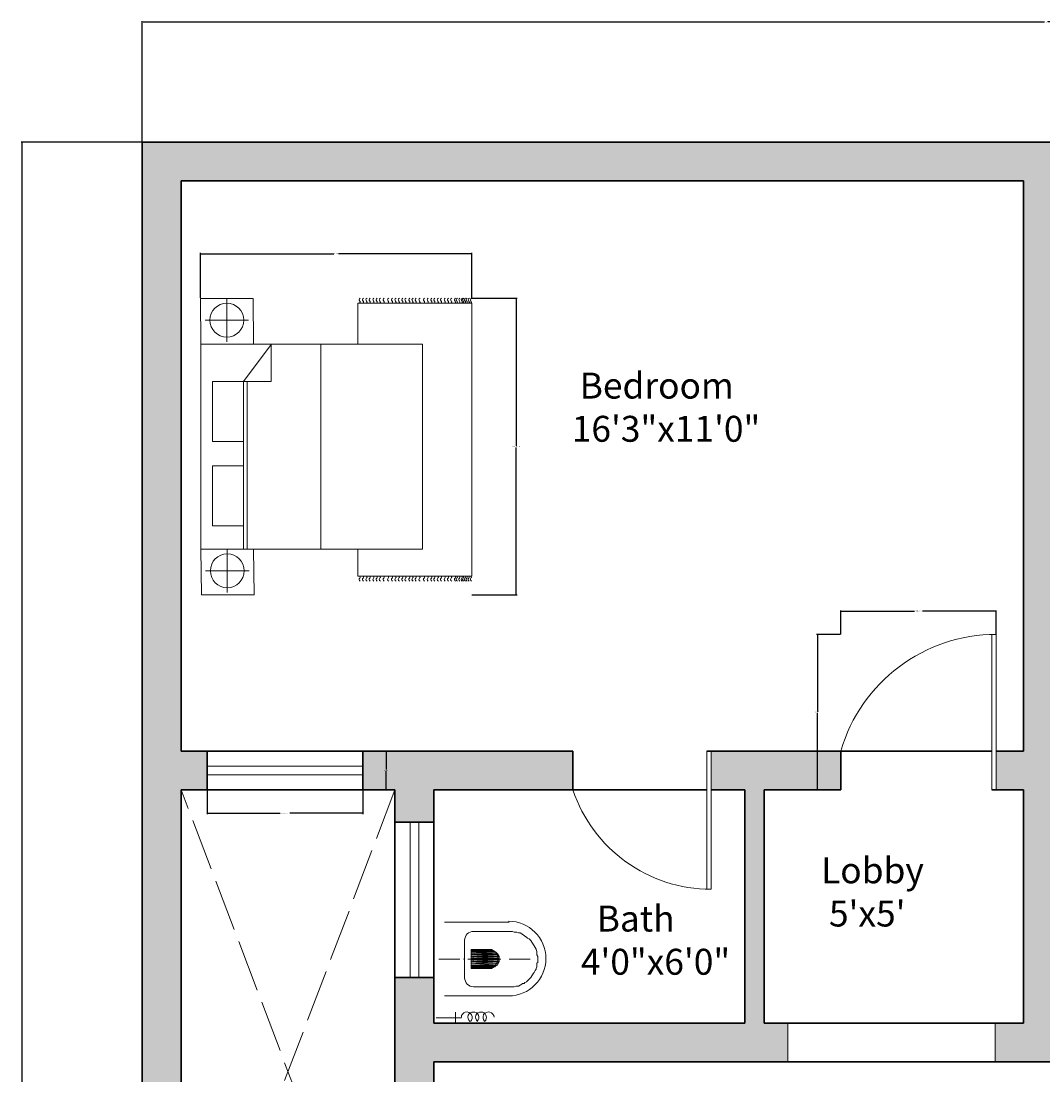
# Model space of a CAD drawing. Units: inches. Extents: x 1752 to 2227, y 6273 to 6884.
# Tile 5 of 6: x 1752 to 1989, y 6640 to 6884. Entities that reach past the tile are written whole.
import ezdxf

# ---------------------------------------------------------------- set-up
doc = ezdxf.new("R2010")
doc.units = ezdxf.units.IN
doc.header["$MEASUREMENT"] = 0
doc.linetypes.add('ACAD_ISO02W100', pattern=[15, 12, -3])
for name, color, linetype, lineweight in [('A-ANNO-DIMS', 2, 'Continuous', 18), ('A-AREA-IDEN', 7, 'Continuous', 18), ('A-DOOR', 3, 'Continuous', 20), ('A-FLOR-FIXT', 8, 'Continuous', 18), ('A-FLOR-VOID', 8, 'ACAD_ISO02W100', 13), ('A-FURN', 8, 'Continuous', 18), ('A-GLAZ', 4, 'Continuous', 18), ('A-WALL', 7, 'Continuous', 35), ('A-WALL-OPNG', 7, 'Continuous', 18)]:
    doc.layers.add(name, color=color, linetype=linetype, lineweight=lineweight)
doc.layers.add('A-WALL-PATT', color=32, linetype='Continuous', lineweight=13, true_color=0xcd6928)
doc.styles.get("Standard").update_dxf_attribs({"font": 'arial.ttf'})
doc.dimstyles.get("Standard").update_dxf_attribs({"dimtxt": 0.18, "dimasz": 0.18, "dimexe": 0.18, "dimexo": 0.0625, "dimgap": 0.09, "dimtad": 0, "dimtih": 1, "dimtoh": 1, "dimdec": 4, "dimzin": 0, "dimdsep": 46, "dimtxsty": 'Standard', "dimcen": 0.09, "dimadec": 0, "dimazin": 0, "dimtfac": 1, "dimtdec": 4, "dimtofl": 0, "dimtmove": 0, "dimatfit": 3, "dimfxl": 1, "dimtolj": 1, "dimtzin": 0, "dimarcsym": 0})

# ---------------------------------------------------------------- blocks, each defined once
blk = doc.blocks.new('BED-DOUBLE-SET')
for p, q in [((5.6, 61.62), (5.6, 51.56)), ((63.65, 61.72), (63.65, 51.66)), ((10.63, 56.59), (0.57, 56.59)), ((68.68, 56.69), (58.62, 56.69)), ((49.39, 52.82), (10.63, 52.82)), ((49.44, 52), (10.63, 52)), ((49.39, 52.82), (58, 46.47)), ((49.44, 52.82), (49.44, 46.47)), ((49.44, 46.47), (58, 46.47)), ((58.05, 34.96), (10.63, 34.96)), ((4.35, 0), (4.35, 26.37)), ((4.35, 26.37), (10.65, 26.37)), ((58.05, 26.37), (67.59, 26.37)), ((67.59, 26.37), (67.59, 0)), ((67.59, 0), (4.35, 0))]:
    blk.add_line(p, q)
for points in [[(0, 50.39), (10.63, 50.5), (10.63, 62.68), (0, 62.58)], [(58.05, 62.68), (58.05, 11.37), (10.63, 11.37), (10.63, 62.68)], [(58.05, 50.5), (68.68, 50.6), (68.68, 62.78), (58.05, 62.68)], [(29.88, 59.98), (29.88, 52.82), (15.98, 52.82), (15.98, 59.98)], [(49.44, 59.98), (49.44, 52.82), (35.55, 52.82), (35.55, 59.98)]]:
    blk.add_lwpolyline(points, close=True)
for centre in [(5.6, 56.59), (63.65, 56.69)]:
    blk.add_circle(centre, 3.92)
for points, knots in [([(3.23, 25.84), (3.32, 25.96), (3.52, 26.2), (3.86, 25.96), (4.14, 25.78), (4.29, 25.89), (4.35, 25.94)], [0, 0, 0, 0, 0.400747, 0.791423, 1.067667, 1.29709, 1.29709, 1.29709, 1.29709]), ([(3.23, 25.06), (3.32, 25.18), (3.52, 25.42), (3.86, 25.18), (4.14, 25.01), (4.29, 25.11), (4.35, 25.16)], [0, 0, 0, 0, 0.400747, 0.791423, 1.067667, 1.29709, 1.29709, 1.29709, 1.29709]), ([(3.23, 24.24), (3.32, 24.36), (3.52, 24.6), (3.86, 24.36), (4.14, 24.19), (4.29, 24.3), (4.35, 24.34)], [0, 0, 0, 0, 0.400747, 0.791423, 1.067667, 1.29709, 1.29709, 1.29709, 1.29709]), ([(68.71, 25.84), (68.61, 25.96), (68.42, 26.2), (68.08, 25.96), (67.8, 25.78), (67.65, 25.89), (67.58, 25.94)], [0, 0, 0, 0, 0.400747, 0.791423, 1.067667, 1.29709, 1.29709, 1.29709, 1.29709]), ([(68.71, 25.06), (68.61, 25.18), (68.42, 25.42), (68.08, 25.18), (67.8, 25.01), (67.65, 25.11), (67.58, 25.16)], [0, 0, 0, 0, 0.400747, 0.791423, 1.067667, 1.29709, 1.29709, 1.29709, 1.29709]), ([(68.71, 24.24), (68.61, 24.36), (68.42, 24.6), (68.08, 24.36), (67.8, 24.19), (67.65, 24.3), (67.58, 24.34)], [0, 0, 0, 0, 0.400747, 0.791423, 1.067667, 1.29709, 1.29709, 1.29709, 1.29709]), ([(3.23, 23.51), (3.32, 23.63), (3.52, 23.87), (3.86, 23.63), (4.14, 23.46), (4.29, 23.57), (4.35, 23.62)], [0, 0, 0, 0, 0.400747, 0.791423, 1.067667, 1.29709, 1.29709, 1.29709, 1.29709]), ([(3.23, 22.63), (3.32, 22.75), (3.52, 22.99), (3.86, 22.75), (4.14, 22.58), (4.29, 22.69), (4.35, 22.73)], [0, 0, 0, 0, 0.400747, 0.791423, 1.067667, 1.29709, 1.29709, 1.29709, 1.29709]), ([(3.23, 21.88), (3.32, 22), (3.52, 22.24), (3.86, 22), (4.14, 21.83), (4.29, 21.93), (4.35, 21.98)], [0, 0, 0, 0, 0.400747, 0.791423, 1.067667, 1.29709, 1.29709, 1.29709, 1.29709]), ([(68.71, 23.51), (68.61, 23.63), (68.42, 23.87), (68.08, 23.63), (67.8, 23.46), (67.65, 23.57), (67.58, 23.62)], [0, 0, 0, 0, 0.400747, 0.791423, 1.067667, 1.29709, 1.29709, 1.29709, 1.29709]), ([(68.71, 22.63), (68.61, 22.75), (68.42, 22.99), (68.08, 22.75), (67.8, 22.58), (67.65, 22.69), (67.58, 22.73)], [0, 0, 0, 0, 0.400747, 0.791423, 1.067667, 1.29709, 1.29709, 1.29709, 1.29709]), ([(68.71, 21.88), (68.61, 22), (68.42, 22.24), (68.08, 22), (67.8, 21.83), (67.65, 21.93), (67.58, 21.98)], [0, 0, 0, 0, 0.400747, 0.791423, 1.067667, 1.29709, 1.29709, 1.29709, 1.29709]), ([(3.23, 21.15), (3.32, 21.27), (3.52, 21.51), (3.86, 21.27), (4.14, 21.1), (4.29, 21.21), (4.35, 21.25)], [0, 0, 0, 0, 0.400747, 0.791423, 1.067667, 1.29709, 1.29709, 1.29709, 1.29709]), ([(3.23, 20.27), (3.32, 20.39), (3.52, 20.63), (3.86, 20.39), (4.14, 20.22), (4.29, 20.32), (4.35, 20.37)], [0, 0, 0, 0, 0.400747, 0.791423, 1.067667, 1.29709, 1.29709, 1.29709, 1.29709]), ([(68.71, 21.15), (68.61, 21.27), (68.42, 21.51), (68.08, 21.27), (67.8, 21.1), (67.65, 21.21), (67.58, 21.25)], [0, 0, 0, 0, 0.400747, 0.791423, 1.067667, 1.29709, 1.29709, 1.29709, 1.29709]), ([(68.71, 20.27), (68.61, 20.39), (68.42, 20.63), (68.08, 20.39), (67.8, 20.22), (67.65, 20.32), (67.58, 20.37)], [0, 0, 0, 0, 0.400747, 0.791423, 1.067667, 1.29709, 1.29709, 1.29709, 1.29709]), ([(3.23, 19.23), (3.32, 19.35), (3.52, 19.59), (3.86, 19.35), (4.14, 19.18), (4.29, 19.29), (4.35, 19.33)], [0, 0, 0, 0, 0.400747, 0.791423, 1.067667, 1.29709, 1.29709, 1.29709, 1.29709]), ([(3.23, 18.35), (3.32, 18.47), (3.52, 18.71), (3.86, 18.47), (4.14, 18.3), (4.29, 18.4), (4.35, 18.45)], [0, 0, 0, 0, 0.400747, 0.791423, 1.067667, 1.29709, 1.29709, 1.29709, 1.29709]), ([(3.23, 17.53), (3.32, 17.65), (3.52, 17.89), (3.86, 17.65), (4.14, 17.48), (4.29, 17.59), (4.35, 17.64)], [0, 0, 0, 0, 0.400747, 0.791423, 1.067667, 1.29709, 1.29709, 1.29709, 1.29709]), ([(68.71, 19.23), (68.61, 19.35), (68.42, 19.59), (68.08, 19.35), (67.8, 19.18), (67.65, 19.29), (67.58, 19.33)], [0, 0, 0, 0, 0.400747, 0.791423, 1.067667, 1.29709, 1.29709, 1.29709, 1.29709]), ([(68.71, 18.35), (68.61, 18.47), (68.42, 18.71), (68.08, 18.47), (67.8, 18.3), (67.65, 18.4), (67.58, 18.45)], [0, 0, 0, 0, 0.400747, 0.791423, 1.067667, 1.29709, 1.29709, 1.29709, 1.29709]), ([(68.71, 17.53), (68.61, 17.65), (68.42, 17.89), (68.08, 17.65), (67.8, 17.48), (67.65, 17.59), (67.58, 17.64)], [0, 0, 0, 0, 0.400747, 0.791423, 1.067667, 1.29709, 1.29709, 1.29709, 1.29709]), ([(3.23, 16.76), (3.32, 16.88), (3.52, 17.12), (3.86, 16.88), (4.14, 16.71), (4.29, 16.81), (4.35, 16.86)], [0, 0, 0, 0, 0.400747, 0.791423, 1.067667, 1.29709, 1.29709, 1.29709, 1.29709]), ([(3.23, 15.94), (3.32, 16.06), (3.52, 16.3), (3.86, 16.06), (4.14, 15.89), (4.29, 16), (4.35, 16.04)], [0, 0, 0, 0, 0.400747, 0.791423, 1.067667, 1.29709, 1.29709, 1.29709, 1.29709]), ([(3.23, 15.21), (3.32, 15.33), (3.52, 15.57), (3.86, 15.33), (4.14, 15.16), (4.29, 15.27), (4.35, 15.32)], [0, 0, 0, 0, 0.400747, 0.791423, 1.067667, 1.29709, 1.29709, 1.29709, 1.29709]), ([(68.71, 16.76), (68.61, 16.88), (68.42, 17.12), (68.08, 16.88), (67.8, 16.71), (67.65, 16.81), (67.58, 16.86)], [0, 0, 0, 0, 0.400747, 0.791423, 1.067667, 1.29709, 1.29709, 1.29709, 1.29709]), ([(68.71, 15.94), (68.61, 16.06), (68.42, 16.3), (68.08, 16.06), (67.8, 15.89), (67.65, 16), (67.58, 16.04)], [0, 0, 0, 0, 0.400747, 0.791423, 1.067667, 1.29709, 1.29709, 1.29709, 1.29709]), ([(68.71, 15.21), (68.61, 15.33), (68.42, 15.57), (68.08, 15.33), (67.8, 15.16), (67.65, 15.27), (67.58, 15.32)], [0, 0, 0, 0, 0.400747, 0.791423, 1.067667, 1.29709, 1.29709, 1.29709, 1.29709]), ([(3.23, 14.33), (3.32, 14.45), (3.52, 14.69), (3.86, 14.45), (4.14, 14.28), (4.29, 14.39), (4.35, 14.43)], [0, 0, 0, 0, 0.400747, 0.791423, 1.067667, 1.29709, 1.29709, 1.29709, 1.29709]), ([(3.23, 13.58), (3.32, 13.7), (3.52, 13.94), (3.86, 13.7), (4.14, 13.53), (4.29, 13.63), (4.35, 13.68)], [0, 0, 0, 0, 0.400747, 0.791423, 1.067667, 1.29709, 1.29709, 1.29709, 1.29709]), ([(3.23, 12.85), (3.32, 12.97), (3.52, 13.21), (3.86, 12.97), (4.14, 12.8), (4.29, 12.9), (4.35, 12.95)], [0, 0, 0, 0, 0.400747, 0.791423, 1.067667, 1.29709, 1.29709, 1.29709, 1.29709]), ([(3.23, 11.97), (3.32, 12.09), (3.52, 12.33), (3.86, 12.09), (4.14, 11.92), (4.29, 12.02), (4.35, 12.07)], [0, 0, 0, 0, 0.400747, 0.791423, 1.067667, 1.29709, 1.29709, 1.29709, 1.29709]), ([(68.71, 14.33), (68.61, 14.45), (68.42, 14.69), (68.08, 14.45), (67.8, 14.28), (67.65, 14.39), (67.58, 14.43)], [0, 0, 0, 0, 0.400747, 0.791423, 1.067667, 1.29709, 1.29709, 1.29709, 1.29709]), ([(68.71, 13.58), (68.61, 13.7), (68.42, 13.94), (68.08, 13.7), (67.8, 13.53), (67.65, 13.63), (67.58, 13.68)], [0, 0, 0, 0, 0.400747, 0.791423, 1.067667, 1.29709, 1.29709, 1.29709, 1.29709]), ([(68.71, 12.85), (68.61, 12.97), (68.42, 13.21), (68.08, 12.97), (67.8, 12.8), (67.65, 12.9), (67.58, 12.95)], [0, 0, 0, 0, 0.400747, 0.791423, 1.067667, 1.29709, 1.29709, 1.29709, 1.29709]), ([(68.71, 11.97), (68.61, 12.09), (68.42, 12.33), (68.08, 12.09), (67.8, 11.92), (67.65, 12.02), (67.58, 12.07)], [0, 0, 0, 0, 0.400747, 0.791423, 1.067667, 1.29709, 1.29709, 1.29709, 1.29709]), ([(3.23, 10.93), (3.32, 11.05), (3.52, 11.29), (3.86, 11.05), (4.14, 10.88), (4.29, 10.99), (4.35, 11.03)], [0, 0, 0, 0, 0.400747, 0.791423, 1.067667, 1.29709, 1.29709, 1.29709, 1.29709]), ([(3.23, 10.05), (3.32, 10.17), (3.52, 10.41), (3.86, 10.17), (4.14, 10), (4.29, 10.1), (4.35, 10.15)], [0, 0, 0, 0, 0.400747, 0.791423, 1.067667, 1.29709, 1.29709, 1.29709, 1.29709]), ([(68.71, 10.93), (68.61, 11.05), (68.42, 11.29), (68.08, 11.05), (67.8, 10.88), (67.65, 10.99), (67.58, 11.03)], [0, 0, 0, 0, 0.400747, 0.791423, 1.067667, 1.29709, 1.29709, 1.29709, 1.29709]), ([(68.71, 10.05), (68.61, 10.17), (68.42, 10.41), (68.08, 10.17), (67.8, 10), (67.65, 10.1), (67.58, 10.15)], [0, 0, 0, 0, 0.400747, 0.791423, 1.067667, 1.29709, 1.29709, 1.29709, 1.29709]), ([(3.23, 9.23), (3.32, 9.35), (3.52, 9.59), (3.86, 9.35), (4.14, 9.18), (4.29, 9.29), (4.35, 9.34)], [0, 0, 0, 0, 0.400747, 0.791423, 1.067667, 1.29709, 1.29709, 1.29709, 1.29709]), ([(3.23, 8.54), (3.32, 8.66), (3.52, 8.9), (3.86, 8.66), (4.14, 8.49), (4.29, 8.6), (4.35, 8.65)], [0, 0, 0, 0, 0.400747, 0.791423, 1.067667, 1.29709, 1.29709, 1.29709, 1.29709]), ([(3.23, 7.73), (3.32, 7.85), (3.52, 8.09), (3.86, 7.85), (4.14, 7.68), (4.29, 7.78), (4.35, 7.83)], [0, 0, 0, 0, 0.400747, 0.791423, 1.067667, 1.29709, 1.29709, 1.29709, 1.29709]), ([(68.71, 9.23), (68.61, 9.35), (68.42, 9.59), (68.08, 9.35), (67.8, 9.18), (67.65, 9.29), (67.58, 9.34)], [0, 0, 0, 0, 0.400747, 0.791423, 1.067667, 1.29709, 1.29709, 1.29709, 1.29709]), ([(68.71, 8.54), (68.61, 8.66), (68.42, 8.9), (68.08, 8.66), (67.8, 8.49), (67.65, 8.6), (67.58, 8.65)], [0, 0, 0, 0, 0.400747, 0.791423, 1.067667, 1.29709, 1.29709, 1.29709, 1.29709]), ([(68.71, 7.73), (68.61, 7.85), (68.42, 8.09), (68.08, 7.85), (67.8, 7.68), (67.65, 7.78), (67.58, 7.83)], [0, 0, 0, 0, 0.400747, 0.791423, 1.067667, 1.29709, 1.29709, 1.29709, 1.29709]), ([(3.23, 7), (3.32, 7.12), (3.52, 7.36), (3.86, 7.12), (4.14, 6.95), (4.29, 7.05), (4.35, 7.1)], [0, 0, 0, 0, 0.400747, 0.791423, 1.067667, 1.29709, 1.29709, 1.29709, 1.29709]), ([(3.23, 6.12), (3.32, 6.24), (3.52, 6.48), (3.86, 6.24), (4.14, 6.07), (4.29, 6.17), (4.35, 6.22)], [0, 0, 0, 0, 0.400747, 0.791423, 1.067667, 1.29709, 1.29709, 1.29709, 1.29709]), ([(3.23, 5.37), (3.32, 5.49), (3.52, 5.73), (3.86, 5.49), (4.14, 5.31), (4.29, 5.42), (4.35, 5.47)], [0, 0, 0, 0, 0.400747, 0.791423, 1.067667, 1.29709, 1.29709, 1.29709, 1.29709]), ([(3.23, 4.64), (3.32, 4.76), (3.52, 5), (3.86, 4.76), (4.14, 4.59), (4.29, 4.69), (4.35, 4.74)], [0, 0, 0, 0, 0.400747, 0.791423, 1.067667, 1.29709, 1.29709, 1.29709, 1.29709]), ([(68.71, 7), (68.61, 7.12), (68.42, 7.36), (68.08, 7.12), (67.8, 6.95), (67.65, 7.05), (67.58, 7.1)], [0, 0, 0, 0, 0.400747, 0.791423, 1.067667, 1.29709, 1.29709, 1.29709, 1.29709]), ([(68.71, 6.12), (68.61, 6.24), (68.42, 6.48), (68.08, 6.24), (67.8, 6.07), (67.65, 6.17), (67.58, 6.22)], [0, 0, 0, 0, 0.400747, 0.791423, 1.067667, 1.29709, 1.29709, 1.29709, 1.29709]), ([(68.71, 5.37), (68.61, 5.49), (68.42, 5.73), (68.08, 5.49), (67.8, 5.31), (67.65, 5.42), (67.58, 5.47)], [0, 0, 0, 0, 0.400747, 0.791423, 1.067667, 1.29709, 1.29709, 1.29709, 1.29709]), ([(68.71, 4.64), (68.61, 4.76), (68.42, 5), (68.08, 4.76), (67.8, 4.59), (67.66, 4.69), (67.59, 4.73)], [0, 0, 0, 0, 0.400747, 0.791423, 1.067667, 1.283686, 1.283686, 1.283686, 1.283686]), ([(3.23, 3.75), (3.32, 3.88), (3.52, 4.12), (3.86, 3.88), (4.14, 3.7), (4.29, 3.81), (4.35, 3.86)], [0, 0, 0, 0, 0.400747, 0.791423, 1.067667, 1.29709, 1.29709, 1.29709, 1.29709]), ([(3.23, 3.33), (3.32, 3.45), (3.52, 3.7), (3.86, 3.45), (4.14, 3.27), (4.29, 3.38), (4.35, 3.43)], [0, 0, 0, 0, 0.407265, 0.802015, 1.07826, 1.307683, 1.307683, 1.307683, 1.307683]), ([(3.23, 2.76), (3.32, 2.88), (3.52, 3.12), (3.86, 2.88), (4.14, 2.71), (4.29, 2.81), (4.35, 2.86)], [0, 0, 0, 0, 0.400747, 0.791423, 1.067667, 1.29709, 1.29709, 1.29709, 1.29709]), ([(3.23, 2.19), (3.32, 2.31), (3.52, 2.55), (3.86, 2.31), (4.14, 2.13), (4.29, 2.24), (4.35, 2.29)], [0, 0, 0, 0, 0.400747, 0.791423, 1.067667, 1.29709, 1.29709, 1.29709, 1.29709]), ([(68.71, 3.75), (68.61, 3.88), (68.42, 4.12), (68.08, 3.88), (67.8, 3.7), (67.66, 3.81), (67.59, 3.85)], [0, 0, 0, 0, 0.400747, 0.791423, 1.067667, 1.283686, 1.283686, 1.283686, 1.283686]), ([(68.71, 3.33), (68.61, 3.45), (68.42, 3.69), (68.08, 3.45), (67.8, 3.28), (67.66, 3.38), (67.59, 3.42)], [0, 0, 0, 0, 0.402903, 0.794912, 1.071156, 1.287177, 1.287177, 1.287177, 1.287177]), ([(68.71, 2.73), (68.61, 2.85), (68.42, 3.09), (68.08, 2.85), (67.8, 2.68), (67.66, 2.78), (67.59, 2.83)], [0, 0, 0, 0, 0.400747, 0.791423, 1.067667, 1.283686, 1.283686, 1.283686, 1.283686]), ([(3.23, 1.88), (3.32, 2), (3.52, 2.24), (3.86, 2), (4.14, 1.82), (4.29, 1.93), (4.35, 1.98)], [0, 0, 0, 0, 0.400747, 0.791423, 1.067667, 1.29709, 1.29709, 1.29709, 1.29709]), ([(3.23, 1.46), (3.32, 1.58), (3.52, 1.82), (3.86, 1.58), (4.14, 1.41), (4.29, 1.51), (4.35, 1.56)], [0, 0, 0, 0, 0.400747, 0.791423, 1.067667, 1.29709, 1.29709, 1.29709, 1.29709]), ([(3.23, 1.06), (3.32, 1.18), (3.52, 1.42), (3.86, 1.18), (4.14, 1.01), (4.29, 1.11), (4.35, 1.16)], [0, 0, 0, 0, 0.400747, 0.791423, 1.067667, 1.29709, 1.29709, 1.29709, 1.29709]), ([(3.23, 0.57), (3.32, 0.7), (3.52, 0.94), (3.86, 0.7), (4.14, 0.52), (4.29, 0.63), (4.35, 0.68)], [0, 0, 0, 0, 0.400747, 0.791423, 1.067667, 1.29709, 1.29709, 1.29709, 1.29709]), ([(3.23, 0.07), (3.32, 0.19), (3.52, 0.43), (3.86, 0.19), (4.14, 0.02), (4.29, 0.13), (4.35, 0.18)], [0, 0, 0, 0, 0.400747, 0.791423, 1.067667, 1.29709, 1.29709, 1.29709, 1.29709]), ([(68.71, 1.43), (68.61, 1.55), (68.42, 1.79), (68.08, 1.55), (67.8, 1.38), (67.65, 1.48), (67.58, 1.53)], [0, 0, 0, 0, 0.400747, 0.791423, 1.067667, 1.29709, 1.29709, 1.29709, 1.29709]), ([(68.71, 1.03), (68.61, 1.15), (68.42, 1.39), (68.08, 1.15), (67.8, 0.98), (67.65, 1.09), (67.58, 1.13)], [0, 0, 0, 0, 0.400747, 0.791423, 1.067667, 1.29709, 1.29709, 1.29709, 1.29709]), ([(68.71, 0.55), (68.61, 0.67), (68.42, 0.91), (68.08, 0.67), (67.8, 0.5), (67.65, 0.6), (67.58, 0.65)], [0, 0, 0, 0, 0.400747, 0.791423, 1.067667, 1.29709, 1.29709, 1.29709, 1.29709]), ([(68.71, 0.07), (68.61, 0.19), (68.42, 0.43), (68.08, 0.19), (67.8, 0.02), (67.65, 0.13), (67.58, 0.18)], [0, 0, 0, 0, 0.400747, 0.791423, 1.067667, 1.29709, 1.29709, 1.29709, 1.29709]), ([(68.71, 2.16), (68.61, 2.28), (68.42, 2.52), (68.08, 2.28), (67.8, 2.11), (67.66, 2.21), (67.59, 2.25)], [0, 0, 0, 0, 0.400747, 0.791423, 1.067667, 1.283686, 1.283686, 1.283686, 1.283686]), ([(68.71, 1.85), (68.61, 1.97), (68.42, 2.21), (68.08, 1.97), (67.8, 1.8), (67.66, 1.9), (67.59, 1.94)], [0, 0, 0, 0, 0.400747, 0.791423, 1.067667, 1.283686, 1.283686, 1.283686, 1.283686])]:
    blk.add_open_spline(points, degree=3, knots=knots)
blk = doc.blocks.new('WC-PLAN')
h = blk.add_hatch(color=256)
h.paths.add_polyline_path([(8.12, 16.94), (13.2, 16.94), (8.12, 17.17)])
h.paths.add_polyline_path([(13.2, 16.94), (8.12, 17.17), (12.82, 17.17)])
h.paths.add_polyline_path([(8.12, 17.17), (12.82, 17.17), (12.44, 17.17)])
h = blk.add_hatch(color=256)
h.paths.add_polyline_path([(8.12, 16.71), (13.58, 16.71), (8.12, 16.94)])
h.paths.add_polyline_path([(13.58, 16.71), (8.12, 16.94), (13.2, 16.94)])
h = blk.add_hatch(color=256)
h.paths.add_polyline_path([(8.12, 16.56), (13.81, 16.56), (8.12, 16.71)])
h.paths.add_polyline_path([(13.81, 16.56), (8.12, 16.71), (13.58, 16.71)])
h = blk.add_hatch(color=256)
h.paths.add_polyline_path([(8.12, 16.18), (14.19, 16.18), (8.12, 16.56)])
h.paths.add_polyline_path([(14.19, 16.18), (8.12, 16.56), (13.81, 16.56)])
h = blk.add_hatch(color=256)
h.paths.add_polyline_path([(8.12, 15.95), (14.34, 15.95), (8.12, 16.18)])
h.paths.add_polyline_path([(14.34, 15.95), (8.12, 16.18), (14.19, 16.18)])
h = blk.add_hatch(color=256)
h.paths.add_polyline_path([(8.12, 15.57), (14.56, 15.57), (8.12, 15.95)])
h.paths.add_polyline_path([(14.56, 15.57), (8.12, 15.95), (14.34, 15.95)])
h = blk.add_hatch(color=256)
h.paths.add_polyline_path([(8.12, 15.19), (14.56, 15.19), (8.12, 15.57)])
h.paths.add_polyline_path([(14.56, 15.19), (8.12, 15.57), (14.56, 15.57)])
h = blk.add_hatch(color=256)
h.paths.add_polyline_path([(8.12, 14.81), (14.56, 14.81), (8.12, 15.19)])
h.paths.add_polyline_path([(14.56, 14.81), (8.12, 15.19), (14.56, 15.19)])
h = blk.add_hatch(color=256)
h.paths.add_polyline_path([(8.12, 14.44), (14.56, 14.44), (8.12, 14.81)])
h.paths.add_polyline_path([(14.56, 14.44), (8.12, 14.81), (14.56, 14.81)])
h = blk.add_hatch(color=256)
h.paths.add_polyline_path([(8.12, 14.06), (14.34, 14.06), (8.12, 14.44)])
h.paths.add_polyline_path([(14.34, 14.06), (8.12, 14.44), (14.56, 14.44)])
h = blk.add_hatch(color=256)
h.paths.add_polyline_path([(8.12, 13.6), (14.19, 13.6), (8.12, 14.06)])
h.paths.add_polyline_path([(14.19, 13.6), (8.12, 14.06), (14.34, 14.06)])
h = blk.add_hatch(color=256)
h.paths.add_polyline_path([(8.12, 13.45), (13.81, 13.45), (8.12, 13.6)])
h.paths.add_polyline_path([(13.81, 13.45), (8.12, 13.6), (14.19, 13.6)])
h = blk.add_hatch(color=256)
h.paths.add_polyline_path([(8.12, 13.22), (13.58, 13.22), (8.12, 13.45)])
h.paths.add_polyline_path([(13.58, 13.22), (8.12, 13.45), (13.81, 13.45)])
h = blk.add_hatch(color=256)
h.paths.add_polyline_path([(8.12, 13.07), (13.2, 13.07), (8.12, 13.22)])
h.paths.add_polyline_path([(13.2, 13.07), (8.12, 13.22), (13.58, 13.22)])
h = blk.add_hatch(color=256)
h.paths.add_polyline_path([(8.12, 12.84), (12.82, 12.84), (8.12, 13.07)])
h.paths.add_polyline_path([(12.82, 12.84), (8.12, 13.07), (13.2, 13.07)])
for points in [[(1.9, 23.54), (16.92, 23.54), (16.92, 23.54)], [(8.72, 21.41), (15.93, 21.41), (15.93, 21.41)], [(15.93, 21.41), (16.69, 21.41), (17.3, 21.41), (17.67, 21.41), (18.05, 21.19), (18.43, 21.19), (18.66, 21.19), (19.04, 21.04), (19.42, 21.04), (19.8, 20.81), (20.03, 20.66), (20.41, 20.43), (20.56, 20.28), (20.94, 20.05), (21.16, 19.82), (21.54, 19.67), (21.77, 19.44), (21.92, 19.29), (22.15, 18.91), (22.3, 18.68), (22.53, 18.3), (22.68, 18.08), (22.91, 17.7), (23.14, 17.32), (23.14, 17.17), (23.29, 16.71), (23.29, 16.33), (23.29, 15.95), (23.52, 15.57), (23.52, 14.97), (23.52, 14.21), (23.29, 14.06), (23.29, 13.6), (23.29, 13.22), (23.14, 12.84), (23.14, 12.69), (22.91, 12.31), (22.68, 11.86), (22.53, 11.7), (22.3, 11.33), (22.15, 11.1), (21.92, 10.72), (21.77, 10.57), (21.54, 10.34), (21.16, 9.96), (20.94, 9.73), (20.56, 9.58), (20.41, 9.35), (20.03, 9.35), (19.8, 9.2), (19.42, 8.97), (19.04, 8.75), (18.66, 8.75), (18.43, 8.75), (18.05, 8.59), (17.67, 8.59), (17.3, 8.59), (16.69, 8.59), (15.93, 8.59)], [(6.6, 19.29), (6.6, 10.57), (6.6, 10.57)], [(8.12, 17.17), (8.12, 12.84), (8.12, 12.84)], [(8.12, 17.17), (12.44, 17.17), (12.44, 17.17)], [(0.61, 14.97), (5.46, 14.97), (5.46, 14.97)], [(6.37, 14.97), (6.37, 15.04), (6.37, 15.04)], [(7.36, 14.97), (14.94, 14.97), (14.94, 14.97)], [(8.57, 15.42), (8.5, 15.42), (8.5, 15.42)], [(8.57, 14.97), (8.5, 15.04), (8.5, 15.04)], [(8.57, 15.42), (8.57, 15.19), (8.57, 14.97)], [(8.57, 14.97), (8.57, 14.81), (8.57, 14.59)], [(16.92, 14.97), (21.77, 14.97), (21.77, 14.97)], [(8.12, 12.84), (12.44, 12.84), (12.44, 12.84)], [(8.57, 14.59), (8.5, 14.59), (8.5, 14.59)], [(8.72, 8.59), (15.93, 8.59), (15.93, 8.59)], [(1.9, 6.47), (16.92, 6.47), (16.92, 6.47)], [(4.48, 2.73), (4.48, 0), (4.48, 0)], [(0, 1.37), (5.84, 1.37), (5.84, 1.37)]]:
    blk.add_lwpolyline(points)
for points in [[(8.12, 16.94), (13.2, 16.94), (8.12, 17.17)], [(13.2, 16.94), (8.12, 17.17), (12.82, 17.17)], [(8.12, 17.17), (12.82, 17.17), (12.44, 17.17)], [(12.82, 17.17), (8.12, 17.17), (8.12, 17.17)], [(8.12, 16.71), (13.58, 16.71), (8.12, 16.94)], [(13.58, 16.71), (8.12, 16.94), (13.2, 16.94)], [(8.12, 16.56), (13.81, 16.56), (8.12, 16.71)], [(13.81, 16.56), (8.12, 16.71), (13.58, 16.71)], [(8.12, 16.18), (14.19, 16.18), (8.12, 16.56)], [(14.19, 16.18), (8.12, 16.56), (13.81, 16.56)], [(8.12, 15.95), (14.34, 15.95), (8.12, 16.18)], [(14.34, 15.95), (8.12, 16.18), (14.19, 16.18)], [(8.12, 15.57), (14.56, 15.57), (8.12, 15.95)], [(14.56, 15.57), (8.12, 15.95), (14.34, 15.95)], [(8.12, 15.19), (14.56, 15.19), (8.12, 15.57)], [(14.56, 15.19), (8.12, 15.57), (14.56, 15.57)], [(8.12, 14.81), (14.56, 14.81), (8.12, 15.19)], [(14.56, 14.81), (8.12, 15.19), (14.56, 15.19)], [(8.12, 14.44), (14.56, 14.44), (8.12, 14.81)], [(14.56, 14.44), (8.12, 14.81), (14.56, 14.81)], [(8.12, 14.06), (14.34, 14.06), (8.12, 14.44)], [(14.34, 14.06), (8.12, 14.44), (14.56, 14.44)], [(8.12, 13.6), (14.19, 13.6), (8.12, 14.06)], [(14.19, 13.6), (8.12, 14.06), (14.34, 14.06)], [(8.12, 13.45), (13.81, 13.45), (8.12, 13.6)], [(13.81, 13.45), (8.12, 13.6), (14.19, 13.6)], [(8.12, 13.22), (13.58, 13.22), (8.12, 13.45)], [(13.58, 13.22), (8.12, 13.45), (13.81, 13.45)], [(8.12, 13.07), (13.2, 13.07), (8.12, 13.22)], [(13.2, 13.07), (8.12, 13.22), (13.58, 13.22)], [(8.12, 12.84), (12.82, 12.84), (8.12, 13.07)], [(12.82, 12.84), (8.12, 13.07), (13.2, 13.07)], [(8.12, 12.84), (12.44, 12.84)], [(12.44, 12.84), (8.12, 12.84), (12.82, 12.84)]]:
    blk.add_lwpolyline(points, close=True)
for points, knots in [([(16.76, 6.47), (21.54, 6.47), (25.41, 10.34), (25.41, 15.12), (25.41, 15.12), (25.41, 19.9), (21.54, 23.77), (16.76, 23.77)], [0, 0, 0, 0, 0.125, 0.125, 0.125, 0.125001, 1, 1, 1, 1]), ([(12.29, 13.07), (13.43, 13.07), (14.34, 13.98), (14.34, 15.12), (14.34, 15.12), (14.34, 16.26), (13.43, 17.17), (12.29, 17.17)], [0, 0, 0, 0, 0.125, 0.125, 0.125, 0.125001, 1, 1, 1, 1]), ([(7.97, 0.53), (8.34, 0.91), (8.5, 1.59), (8.19, 2.05), (8.19, 2.05), (7.89, 2.58), (7.36, 2.88), (6.75, 2.73), (6.75, 2.73), (6.22, 2.58), (5.84, 2.05), (5.84, 1.52)], [0, 0, 0, 0, 0.083333, 0.083333, 0.083333, 0.083334, 0.166667, 0.166667, 0.166667, 0.166668, 1, 1, 1, 1]), ([(9.48, 0.61), (9.86, 0.91), (10.01, 1.52), (9.79, 1.97), (9.79, 1.97), (9.63, 2.43), (9.1, 2.73), (8.65, 2.73), (8.65, 2.73), (8.12, 2.73), (7.66, 2.43), (7.43, 1.97), (7.43, 1.97), (7.28, 1.44), (7.43, 0.91), (7.81, 0.53)], [0, 0, 0, 0, 0.0625, 0.0625, 0.0625, 0.062501, 0.125, 0.125, 0.125, 0.125001, 0.1875, 0.1875, 0.1875, 0.187501, 1, 1, 1, 1]), ([(11.23, 0.53), (11.61, 0.91), (11.76, 1.44), (11.53, 1.97), (11.53, 1.97), (11.38, 2.43), (10.92, 2.73), (10.39, 2.73), (10.39, 2.73), (9.86, 2.73), (9.41, 2.43), (9.18, 1.97), (9.18, 1.97), (9.03, 1.44), (9.18, 0.91), (9.56, 0.53)], [0, 0, 0, 0, 0.0625, 0.0625, 0.0625, 0.062501, 0.125, 0.125, 0.125, 0.125001, 0.1875, 0.1875, 0.1875, 0.187501, 1, 1, 1, 1]), ([(13.43, 1.52), (13.43, 2.05), (12.97, 2.58), (12.44, 2.73), (12.44, 2.73), (11.91, 2.88), (11.3, 2.58), (11, 2.12), (11, 2.12), (10.77, 1.59), (10.85, 0.99), (11.23, 0.61)], [0, 0, 0, 0, 0.083333, 0.083333, 0.083333, 0.083334, 0.166667, 0.166667, 0.166667, 0.166668, 1, 1, 1, 1])]:
    blk.add_open_spline(points, degree=3, knots=knots)
for points in [[(8.65, 21.41), (7.51, 21.41), (6.6, 20.5), (6.6, 19.37)], [(6.6, 10.64), (6.6, 9.5), (7.51, 8.59), (8.65, 8.59)]]:
    blk.add_open_spline(points, degree=3)
blk = doc.blocks.new('DOOR-SINGLE-36IN')
for p, q in [((35, 36), (35, 0)), ((36, 0), (36, 36)), ((36, 0), (35, 0))]:
    blk.add_line(p, q)
blk.add_arc((36, -1.5), 37.5, 90, 163.7398)
blk = doc.blocks.new('DOOR-SINGLE-32IN')
for p, q in [((32, 32), (31, 32)), ((31, 0), (31, 32)), ((32, 32), (32, 0))]:
    blk.add_line(p, q)
blk.add_arc((32, 33.76), 33.76, 198.5866, 270)
blk = doc.blocks.new('WINDOW-36IN')
for p, q in [((36, 9), (0, 9)), ((36, 5.5), (0, 5.5)), ((0, 3.5), (36, 3.5)), ((0, 0), (36, 0))]:
    blk.add_line(p, q)
blk = doc.blocks.new('*D14')
at = {"layer": 'A-ANNO-DIMS', "color": 0, "lineweight": -2, "transparency": 16777216}
for p, q in [((1856.48, 6819.77), (1866.91, 6819.77)), ((1866.73, 6819.59), (1866.73, 6785.59)), ((1866.73, 6751.24), (1866.73, 6785.23)), ((1856.48, 6751.06), (1866.91, 6751.06))]:
    blk.add_line(p, q, dxfattribs=at)
at = {"layer": 'A-ANNO-DIMS', "color": 0, "transparency": 16777216}
for points in [[(1866.7, 6819.59), (1866.76, 6819.59), (1866.73, 6819.77)], [(1866.7, 6751.24), (1866.76, 6751.24), (1866.73, 6751.06)]]:
    blk.add_solid(points, dxfattribs=at)
at = {"layer": 'Defpoints', "color": 0, "transparency": 16777216}
for p in [(1856.42, 6819.77), (1866.73, 6819.77), (1856.42, 6751.06)]:
    blk.add_point(p, dxfattribs=at)
at = {"layer": 'A-ANNO-DIMS', "color": 0, "transparency": 16777216, "insert": (1866.73, 6785.41), "char_height": 0.18, "attachment_point": 5}
blk.add_mtext('\\A1;BED SET 69 TYP.', dxfattribs=at)
blk = doc.blocks.new('*D15')
at = {"layer": 'A-ANNO-DIMS', "color": 0, "lineweight": -2, "transparency": 16777216}
for p, q in [((1793.64, 6819.83), (1793.64, 6830.25)), ((1793.82, 6830.07), (1824.5, 6830.07)), ((1856.24, 6830.07), (1825.56, 6830.07)), ((1856.42, 6819.83), (1856.42, 6830.25))]:
    blk.add_line(p, q, dxfattribs=at)
at = {"layer": 'A-ANNO-DIMS', "color": 0, "transparency": 16777216}
for points in [[(1793.82, 6830.1), (1793.82, 6830.04), (1793.64, 6830.07)], [(1856.24, 6830.1), (1856.24, 6830.04), (1856.42, 6830.07)]]:
    blk.add_solid(points, dxfattribs=at)
at = {"layer": 'Defpoints', "color": 0, "transparency": 16777216}
for p in [(1793.64, 6830.07), (1793.64, 6819.77), (1856.42, 6819.77)]:
    blk.add_point(p, dxfattribs=at)
at = {"layer": 'A-ANNO-DIMS', "color": 0, "transparency": 16777216, "insert": (1825.03, 6830.07), "char_height": 0.18, "attachment_point": 5}
blk.add_mtext('\\A1;63 TYP.', dxfattribs=at)
blk = doc.blocks.new('*D18')
at = {"layer": 'A-ANNO-DIMS', "color": 0, "lineweight": -2, "transparency": 16777216}
for p, q in [((1941.84, 6741.98), (1941.84, 6747.49)), ((1977.84, 6741.98), (1977.84, 6747.49)), ((1942.02, 6747.31), (1958.91, 6747.31)), ((1977.66, 6747.31), (1960.78, 6747.31))]:
    blk.add_line(p, q, dxfattribs=at)
at = {"layer": 'A-ANNO-DIMS', "color": 0, "transparency": 16777216}
for points in [[(1942.02, 6747.34), (1942.02, 6747.28), (1941.84, 6747.31)], [(1977.66, 6747.34), (1977.66, 6747.28), (1977.84, 6747.31)]]:
    blk.add_solid(points, dxfattribs=at)
at = {"layer": 'Defpoints', "color": 0, "transparency": 16777216}
for p in [(1977.84, 6747.31), (1941.84, 6741.91), (1977.84, 6741.91)]:
    blk.add_point(p, dxfattribs=at)
at = {"layer": 'A-ANNO-DIMS', "color": 0, "transparency": 16777216, "insert": (1959.84, 6747.31), "char_height": 0.18, "attachment_point": 5}
blk.add_mtext('\\A1;DOOR 36 TYP.', dxfattribs=at)
blk = doc.blocks.new('*D19')
at = {"layer": 'A-ANNO-DIMS', "color": 0, "lineweight": -2, "transparency": 16777216}
for p, q in [((1941.78, 6741.91), (1936.26, 6741.91)), ((1936.44, 6741.73), (1936.44, 6724.1)), ((1936.44, 6706.09), (1936.44, 6723.73)), ((1941.78, 6705.91), (1936.26, 6705.91))]:
    blk.add_line(p, q, dxfattribs=at)
at = {"layer": 'A-ANNO-DIMS', "color": 0, "transparency": 16777216}
for points in [[(1936.41, 6741.73), (1936.47, 6741.73), (1936.44, 6741.91)], [(1936.41, 6706.09), (1936.47, 6706.09), (1936.44, 6705.91)]]:
    blk.add_solid(points, dxfattribs=at)
at = {"layer": 'Defpoints', "color": 0, "transparency": 16777216}
for p in [(1936.44, 6741.91), (1941.84, 6741.91), (1941.84, 6705.91)]:
    blk.add_point(p, dxfattribs=at)
at = {"layer": 'A-ANNO-DIMS', "color": 0, "transparency": 16777216, "insert": (1936.44, 6723.91), "char_height": 0.18, "attachment_point": 5}
blk.add_mtext('\\A1;36 TYP.', dxfattribs=at)
blk = doc.blocks.new('*D22')
at = {"layer": 'A-ANNO-DIMS', "color": 0, "lineweight": -2, "transparency": 16777216}
for p, q in [((1795.2, 6705.85), (1795.2, 6700.33)), ((1831.2, 6705.85), (1831.2, 6700.33)), ((1795.38, 6700.51), (1812.09, 6700.51)), ((1831.02, 6700.51), (1814.32, 6700.51))]:
    blk.add_line(p, q, dxfattribs=at)
at = {"layer": 'A-ANNO-DIMS', "color": 0, "transparency": 16777216}
for points in [[(1795.38, 6700.54), (1795.38, 6700.48), (1795.2, 6700.51)], [(1831.02, 6700.54), (1831.02, 6700.48), (1831.2, 6700.51)]]:
    blk.add_solid(points, dxfattribs=at)
at = {"layer": 'Defpoints', "color": 0, "transparency": 16777216}
for p in [(1795.2, 6705.91), (1831.2, 6705.91), (1831.2, 6700.51)]:
    blk.add_point(p, dxfattribs=at)
at = {"layer": 'A-ANNO-DIMS', "color": 0, "transparency": 16777216, "insert": (1813.2, 6700.51), "char_height": 0.18, "attachment_point": 5}
blk.add_mtext('\\A1;WINDOW 36 TYP.', dxfattribs=at)
blk = doc.blocks.new('*D23')
at = {"layer": 'A-ANNO-DIMS', "color": 0, "lineweight": -2, "transparency": 16777216}
for p, q in [((1831.27, 6714.91), (1836.78, 6714.91)), ((1836.6, 6714.73), (1836.6, 6710.6)), ((1836.6, 6706.09), (1836.6, 6710.23)), ((1831.27, 6705.91), (1836.78, 6705.91))]:
    blk.add_line(p, q, dxfattribs=at)
at = {"layer": 'A-ANNO-DIMS', "color": 0, "transparency": 16777216}
for points in [[(1836.57, 6714.73), (1836.63, 6714.73), (1836.6, 6714.91)], [(1836.57, 6706.09), (1836.63, 6706.09), (1836.6, 6705.91)]]:
    blk.add_solid(points, dxfattribs=at)
at = {"layer": 'Defpoints', "color": 0, "transparency": 16777216}
for p in [(1831.2, 6714.91), (1836.6, 6714.91), (1831.2, 6705.91)]:
    blk.add_point(p, dxfattribs=at)
at = {"layer": 'A-ANNO-DIMS', "color": 0, "transparency": 16777216, "insert": (1836.6, 6710.41), "char_height": 0.18, "attachment_point": 5}
blk.add_mtext('\\A1;9 TYP.', dxfattribs=at)
blk = doc.blocks.new('*D40')
at = {"layer": 'A-ANNO-DIMS', "color": 0, "lineweight": -2, "transparency": 16777216}
for p, q in [((1780.15, 6855.98), (1780.15, 6883.94)), ((1780.33, 6883.76), (1989, 6883.76)), ((2198.47, 6883.76), (1989.8, 6883.76)), ((2198.65, 6855.98), (2198.65, 6883.94))]:
    blk.add_line(p, q, dxfattribs=at)
at = {"layer": 'A-ANNO-DIMS', "color": 0, "transparency": 16777216}
for points in [[(1780.33, 6883.79), (1780.33, 6883.73), (1780.15, 6883.76)], [(2198.47, 6883.79), (2198.47, 6883.73), (2198.65, 6883.76)]]:
    blk.add_solid(points, dxfattribs=at)
at = {"layer": 'Defpoints', "color": 0, "transparency": 16777216}
for p in [(2198.65, 6883.76), (1780.15, 6855.91), (2198.65, 6855.91)]:
    blk.add_point(p, dxfattribs=at)
at = {"layer": 'A-ANNO-DIMS', "color": 0, "transparency": 16777216, "insert": (1989.4, 6883.76), "char_height": 0.18, "attachment_point": 5}
blk.add_mtext('\\A1;418.5', dxfattribs=at)
blk = doc.blocks.new('*D41')
at = {"layer": 'A-ANNO-DIMS', "color": 0, "lineweight": -2, "transparency": 16777216}
for p, q in [((1780.08, 6855.91), (1752.12, 6855.91)), ((1752.3, 6855.73), (1752.3, 6583.1)), ((1752.3, 6310.09), (1752.3, 6582.73)), ((1780.08, 6309.91), (1752.12, 6309.91))]:
    blk.add_line(p, q, dxfattribs=at)
at = {"layer": 'A-ANNO-DIMS', "color": 0, "transparency": 16777216}
for points in [[(1752.27, 6855.73), (1752.33, 6855.73), (1752.3, 6855.91)], [(1752.27, 6310.09), (1752.33, 6310.09), (1752.3, 6309.91)]]:
    blk.add_solid(points, dxfattribs=at)
at = {"layer": 'Defpoints', "color": 0, "transparency": 16777216}
for p in [(1752.3, 6855.91), (1780.15, 6855.91), (1780.15, 6309.91)]:
    blk.add_point(p, dxfattribs=at)
at = {"layer": 'A-ANNO-DIMS', "color": 0, "transparency": 16777216, "insert": (1752.3, 6582.91), "char_height": 0.18, "attachment_point": 5}
blk.add_mtext('\\A1;546', dxfattribs=at)

msp = doc.modelspace()

# ---------------------------------------------------------------- hatches: boundary and pattern name
at = {"layer": 'A-WALL-PATT'}
h = msp.add_hatch(color=256, dxfattribs=at)
h.dxf.hatch_style = 1
h.paths.add_polyline_path([(2198.6473, 6855.914), (1780.1473, 6855.914), (1780.1473, 6309.914), (1824.3861, 6309.914), (1824.3861, 6318.914), (1789.1473, 6318.914), (1789.1473, 6501.914), (1790.1473, 6501.914), (1790.1473, 6510.914), (1789.1473, 6510.914), (1789.1473, 6570.914), (1838.6473, 6570.914), (1838.6473, 6510.914), (1822.1473, 6510.914), (1822.1473, 6501.914), (1921.1473, 6501.914), (1921.1473, 6498.914), (1930.1473, 6498.914), (1930.1473, 6501.914), (1930.1473, 6510.914), (1847.6473, 6510.914), (1847.6473, 6585.039), (1838.6473, 6585.039), (1838.6473, 6575.414), (1789.1473, 6575.414), (1789.1473, 6705.914), (1795.2039, 6705.914), (1795.2039, 6714.914), (1789.1473, 6714.914), (1789.1473, 6846.914), (1984.1473, 6846.914), (1984.1473, 6714.914), (1977.8419, 6714.914), (1977.8419, 6705.914), (1984.1473, 6705.914), (1984.1473, 6651.914), (1977.6147, 6651.914), (1977.6147, 6642.914), (1996.1473, 6642.914), (1996.1473, 6651.914), (1993.1473, 6651.914), (1993.1473, 6846.914), (2125.1473, 6846.914), (2125.1473, 6840.4779), (2129.6473, 6840.4779), (2129.6473, 6846.914), (2189.6473, 6846.914), (2189.6473, 6798.914), (2162.6473, 6798.914), (2162.6473, 6794.414), (2189.6473, 6794.414), (2189.6473, 6710.414), (2175.6868, 6710.414), (2175.6868, 6705.914), (2189.6473, 6705.914), (2189.6473, 6651.914), (2164.6473, 6651.914), (2164.6473, 6642.914), (2189.6473, 6642.914), (2189.6473, 6510.914), (2166.7624, 6510.914), (2166.7624, 6501.914), (2189.6473, 6501.914), (2189.6473, 6318.914), (2173.9269, 6318.914), (2173.9269, 6309.914), (2198.6473, 6309.914)])
h.paths.add_polyline_path([(2023.6785, 6318.914), (1930.1473, 6318.914), (1930.1473, 6321.914), (1921.1473, 6321.914), (1921.1473, 6318.914), (1872.3861, 6318.914), (1872.3861, 6309.914), (2023.6785, 6309.914)], flags=17)
h.paths.add_polyline_path([(2092.7496, 6318.914), (2061.7431, 6318.914), (2061.7431, 6309.914), (2092.7496, 6309.914)], flags=0)
h.paths.add_polyline_path([(1947.0033, 6375.914), (1930.1473, 6375.914), (1930.1473, 6462.914), (1921.1473, 6462.914), (1921.1473, 6357.914), (1930.1473, 6357.914), (1930.1473, 6366.914), (1947.0033, 6366.914)], flags=17)
h.paths.add_polyline_path([(2024.6473, 6432.914), (2015.6473, 6432.914), (2015.6473, 6375.914), (1995.0033, 6375.914), (1995.0033, 6366.914), (2024.6473, 6366.914)], flags=17)
h.paths.add_polyline_path([(2030.6473, 6441.914), (2024.6473, 6441.914), (2024.6473, 6510.914), (2015.6473, 6510.914), (2015.6473, 6432.914), (2024.6473, 6432.914), (2030.6473, 6432.914)], flags=17)
h.paths.add_polyline_path([(2093.6473, 6501.914), (2118.7624, 6501.914), (2118.7624, 6510.914), (2093.6473, 6510.914), (2093.6473, 6603.914), (2084.6473, 6603.914), (2084.6473, 6441.914), (2078.6473, 6441.914), (2078.6473, 6432.914), (2093.6473, 6432.914)], flags=17)
h.paths.add_polyline_path([(2132.6473, 6651.914), (2129.6473, 6651.914), (2129.6473, 6705.914), (2139.6868, 6705.914), (2139.6868, 6710.414), (2129.6473, 6710.414), (2129.6473, 6794.414), (2130.6473, 6794.414), (2130.6473, 6798.914), (2129.6473, 6798.914), (2129.6473, 6804.4779), (2125.1473, 6804.4779), (2125.1473, 6651.914), (2032.1473, 6651.914), (2032.1473, 6642.914), (2084.6473, 6642.914), (2084.6473, 6639.914), (2093.6473, 6639.914), (2093.6473, 6642.914), (2132.6473, 6642.914)], flags=17)
h.paths.add_polyline_path([(1929.6147, 6651.914), (1924.1473, 6651.914), (1924.1473, 6705.914), (1941.8419, 6705.914), (1941.8419, 6714.914), (1911.8299, 6714.914), (1911.8299, 6705.914), (1919.6473, 6705.914), (1919.6473, 6651.914), (1847.6473, 6651.914), (1847.6473, 6662.4635), (1838.6473, 6662.4635), (1838.6473, 6621.039), (1847.6473, 6621.039), (1847.6473, 6642.914), (1929.6147, 6642.914)], flags=17)
h.paths.add_polyline_path([(1879.8299, 6714.914), (1831.2039, 6714.914), (1831.2039, 6705.914), (1838.6473, 6705.914), (1838.6473, 6698.4635), (1847.6473, 6698.4635), (1847.6473, 6705.914), (1879.8299, 6705.914)], flags=17)

# ---------------------------------------------------------------- linework, layer by layer
at = {"layer": 'A-DOOR'}
for p, q in [((1977.8419, 6741.914), (1977.8419, 6705.914)), ((1911.8299, 6682.914), (1911.8299, 6714.914))]:
    msp.add_line(p, q, dxfattribs=at)
at = {"layer": 'A-FLOR-VOID'}
for p, q in [((1838.6473, 6705.914), (1789.1473, 6575.414)), ((1838.6473, 6575.414), (1789.1473, 6705.914))]:
    msp.add_line(p, q, dxfattribs=at)
at = {"layer": 'A-WALL'}
for p, q in [((1780.1473, 6855.914), (2198.6473, 6855.914)), ((1780.1473, 6855.914), (1780.1473, 6309.914)), ((1789.1473, 6846.914), (1789.1473, 6714.914)), ((1789.1473, 6846.914), (1984.1473, 6846.914)), ((1984.1473, 6846.914), (1984.1473, 6714.914)), ((1789.1473, 6714.914), (1879.8299, 6714.914)), ((1795.2039, 6714.914), (1795.2039, 6705.914)), ((1831.2039, 6705.914), (1831.2039, 6714.914)), ((1879.8299, 6714.914), (1879.8299, 6705.914)), ((1910.8299, 6714.914), (1976.8419, 6714.914)), ((1941.8419, 6705.914), (1941.8419, 6714.914)), ((1977.8419, 6714.914), (1984.1473, 6714.914)), ((1789.1473, 6705.914), (1838.6473, 6705.914)), ((1789.1473, 6705.914), (1838.6473, 6705.914)), ((1789.1473, 6705.914), (1789.1473, 6575.414)), ((1838.6473, 6705.914), (1838.6473, 6575.414)), ((1847.6473, 6705.914), (1847.6473, 6651.914)), ((1847.6473, 6705.914), (1910.8299, 6705.914)), ((1847.6473, 6705.914), (1910.8299, 6705.914)), ((1911.8299, 6705.914), (1919.6473, 6705.914)), ((1911.8299, 6705.914), (1919.6473, 6705.914)), ((1919.6473, 6705.914), (1919.6473, 6651.914)), ((1924.1473, 6705.914), (1924.1473, 6651.914)), ((1924.1473, 6705.914), (1941.8419, 6705.914)), ((1924.1473, 6705.914), (1941.8419, 6705.914)), ((1976.8419, 6705.914), (1984.1473, 6705.914)), ((1976.8419, 6705.914), (1984.1473, 6705.914)), ((1984.1473, 6705.914), (1984.1473, 6651.914)), ((1838.6473, 6698.4635), (1847.6473, 6698.4635)), ((1847.6473, 6662.4635), (1838.6473, 6662.4635)), ((1847.6473, 6651.914), (1919.6473, 6651.914)), ((1924.1473, 6651.914), (1984.1473, 6651.914)), ((1847.6473, 6642.914), (1997.1473, 6642.914)), ((1847.6473, 6642.914), (1847.6473, 6510.914))]:
    msp.add_line(p, q, dxfattribs=at)
at = {"layer": 'A-WALL-OPNG'}
for p, q in [((1929.6147, 6642.914), (1929.6147, 6651.914)), ((1929.6147, 6651.914), (1977.6147, 6651.914)), ((1977.6147, 6651.914), (1977.6147, 6642.914)), ((1977.6147, 6642.914), (1929.6147, 6642.914))]:
    msp.add_line(p, q, dxfattribs=at)

# ---------------------------------------------------------------- block references
at = {"layer": 'A-DOOR'}
for name, p in [('DOOR-SINGLE-36IN', (1941.842, 6705.914)), ('DOOR-SINGLE-32IN', (1879.83, 6682.914))]:
    msp.add_blockref(name, p, dxfattribs=at)
at = {"layer": 'A-FLOR-FIXT'}
msp.add_blockref('WC-PLAN', (1848.179, 6651.749), dxfattribs=at)
at = {"layer": 'A-FURN', "rotation": 89.99999999999436}
msp.add_blockref('BED-DOUBLE-SET', (1856.4203, 6751.0557), dxfattribs=at)
at = {"layer": 'A-GLAZ'}
msp.add_blockref('WINDOW-36IN', (1795.204, 6705.914), dxfattribs=at)
at = {"layer": 'A-GLAZ', "rotation": 270.0000000000061}
msp.add_blockref('WINDOW-36IN', (1838.6473, 6698.4634), dxfattribs=at)

# ---------------------------------------------------------------- texts
at = {"layer": 'A-AREA-IDEN', "char_height": 6, "attachment_point": 1}
for s, width, insert in [(' Bedroom\\P16\'3"x11\'0"', 76.857973, (1879.5719, 6802.5335)), ("Lobby\\P 5'x5'", 35.678745, (1937.2865, 6690.2821)), ('  Bath\\P4\'0"x6\'0"', 30.465286, (1881.6815, 6679.1174))]:
    msp.add_mtext_dynamic_manual_height_columns(s, width=width, gutter_width=30, heights=[0], dxfattribs=dict(at, insert=insert))

# ---------------------------------------------------------------- dimensions: what is measured, and where the dimension line sits
at = {"layer": 'A-ANNO-DIMS'}
dim = msp.add_linear_dim(base=(2198.6473, 6883.764), p1=(1780.1473, 6855.914), p2=(2198.6473, 6855.914), dimstyle='Standard', override={"dimdec": 1, "dimlfac": 1, "dimrnd": 0, "dimzin": 0, "dimdsep": 46, "dimlunit": 2}, dxfattribs=at)
dim.commit()
dim.dimension.update_dxf_attribs({"geometry": '*D40', "text_midpoint": (1989.3973, 6883.764)})
dim = msp.add_linear_dim(base=(1752.2973, 6855.914), p1=(1780.1473, 6309.914), p2=(1780.1473, 6855.914), angle=90, dimstyle='Standard', override={"dimdec": 0, "dimlfac": 1, "dimrnd": 0, "dimzin": 0, "dimdsep": 46, "dimlunit": 2}, dxfattribs=at)
dim.commit()
dim.dimension.update_dxf_attribs({"geometry": '*D41', "text_midpoint": (1752.2973, 6582.914)})
for base, p1, p2, angle, text, picture, middle in [((1793.6363, 6830.0723), (1856.4198, 6819.7658), (1793.6363, 6819.7658), 180, '<> TYP.', '*D15', (1825.028, 6830.0723)), ((1866.7263, 6819.7658), (1856.4198, 6751.0558), (1856.4198, 6819.7658), 90, 'BED SET <> TYP.', '*D14', (1866.7263, 6785.4108)), ((1936.4419, 6741.914), (1941.8419, 6705.914), (1941.8419, 6741.914), 90, '<> TYP.', '*D19', (1936.4419, 6723.914)), ((1836.6039, 6714.914), (1831.2039, 6705.914), (1831.2039, 6714.914), 90, '<> TYP.', '*D23', (1836.6039, 6710.414))]:
    dim = msp.add_linear_dim(base=base, p1=p1, p2=p2, angle=angle, text=text, dimstyle='Standard', override={"dimdec": 0, "dimlfac": 1, "dimrnd": 0, "dimzin": 0, "dimdsep": 46, "dimlunit": 2}, dxfattribs=at)
    dim.commit()
    dim.dimension.update_dxf_attribs({"geometry": picture, "text_midpoint": middle})
for base, p1, p2, text, picture, middle in [((1977.8419, 6747.314), (1941.8419, 6741.914), (1977.8419, 6741.914), 'DOOR <> TYP.', '*D18', (1959.8419, 6747.314)), ((1831.2039, 6700.514), (1795.2039, 6705.914), (1831.2039, 6705.914), 'WINDOW <> TYP.', '*D22', (1813.2039, 6700.514))]:
    dim = msp.add_linear_dim(base=base, p1=p1, p2=p2, text=text, dimstyle='Standard', override={"dimdec": 0, "dimlfac": 1, "dimrnd": 0, "dimzin": 0, "dimdsep": 46, "dimlunit": 2}, dxfattribs=at)
    dim.commit()
    dim.dimension.update_dxf_attribs({"geometry": picture, "text_midpoint": middle})

doc.saveas('drawing.dxf')
